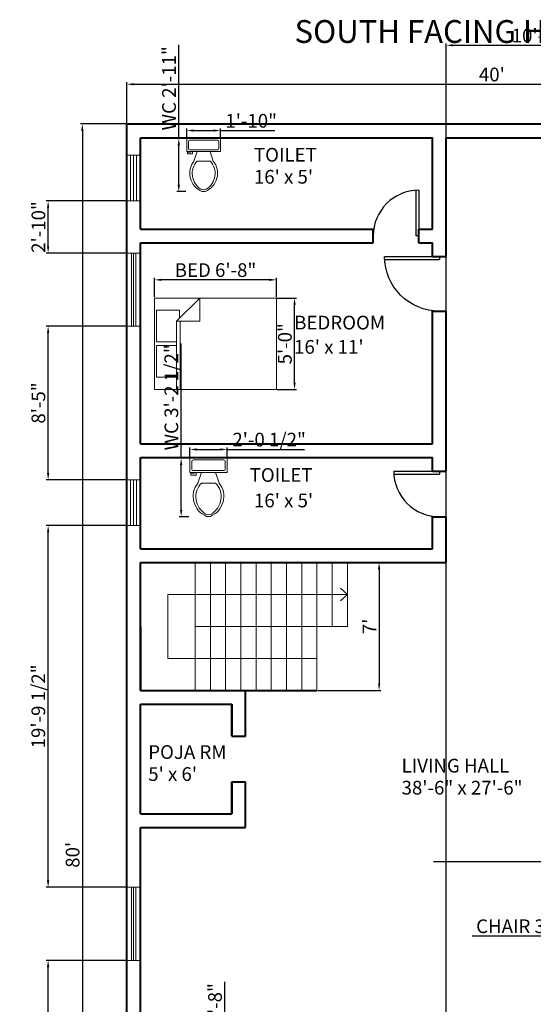
# Model space of a CAD drawing. Units: inches. Extents: x 2383 to 6214, y 970 to 3250.
# Tile 3 of 4: x 2383 to 2721, y 1500 to 2147. Entities that reach past the tile are written whole.
import ezdxf

# ---------------------------------------------------------------- set-up
doc = ezdxf.new("R2010")
doc.units = ezdxf.units.IN
for name, color, linetype, lineweight in [('A-ANNO-DIMS', 2, 'Continuous', 18), ('A-ANNO-TEXT', 7, 'Continuous', 18), ('A-AREA-IDEN', 7, 'Continuous', 18), ('A-DOOR', 4, 'Continuous', 25), ('A-FLOR-FIXT', 8, 'Continuous', 18), ('A-FLOR-STRS', 7, 'Continuous', 20), ('A-FURN', 8, 'Continuous', 18), ('A-GLAZ', 4, 'Continuous', 18), ('A-WALL', 7, 'Continuous', 40)]:
    doc.layers.add(name, color=color, linetype=linetype, lineweight=lineweight)
doc.styles.get("Standard").update_dxf_attribs({"font": 'arial.ttf'})
doc.dimstyles.new('ISO-25', dxfattribs={"dimtxt": 9, "dimasz": 4.5, "dimexe": 1.25, "dimexo": 0.625, "dimtad": 1, "dimdec": 0, "dimlunit": 3, "dimtxsty": 'Standard', "dimcen": 2.5, "dimadec": 0, "dimazin": 0, "dimtfac": 1, "dimtdec": 0, "dimtmove": 0, "dimatfit": 3, "dimfxl": 1, "dimarcsym": 0})

# ---------------------------------------------------------------- blocks, each defined once
blk = doc.blocks.new('Toilet - top')
for p, q in [((9.5, -6), (9.5, -2)), ((-10, -8.5), (-8, -8.5)), ((-10, -9.5), (-10, -8.5)), ((-7, -9.5), (-10, -9.5)), ((-8, -8.5), (-8, -8)), ((-7, -8), (-7, -9.5)), ((-4, -8), (-6, -14)), ((4, -8), (6, -14)), ((4, -14), (-4, -14))]:
    blk.add_line(p, q)
blk.add_lwpolyline([(10.5, -8), (10.5, 0), (-10.5, 0), (-10.5, -8)], close=True)
for points in [[(-9.5, -2), (-9.5, -6)], [(8.5, -1), (-8.5, -1)], [(-8.5, -7), (8.5, -7)]]:
    blk.add_lwpolyline(points)
for centre, radius, start, end in [((-8.62, -1.88), 0.884, 81.8699, 188.1301), ((8.62, -1.88), 0.884, 351.8699, 98.1301), ((-8.62, -6.12), 0.884, 171.8699, 278.1301), ((8.62, -6.12), 0.884, 261.8699, 8.1301), ((3.52, -21.58), 12.17, 141.4691, 247.9714), ((4.2, -21.82), 11.33, 136.3677, 238.9468), ((-3.52, -21.58), 12.17, 292.0284, 38.5307), ((-4.2, -21.82), 11.33, 301.053, 43.6321), ((0, -27.88), 4, 245.7318, 294.2682), ((0, -29), 4, 254.8605, 285.1395)]:
    blk.add_arc(centre, radius, start, end)
blk = doc.blocks.new('Bed - Queen')
for p, q in [((0, -80.00003), (0, 0)), ((0, 0), (59.99999, 0)), ((59.99999, 0), (59.99999, -80.00003)), ((7.99999, -1.2), (28.79998, -1.2)), ((7.99999, -14.4), (7.99999, -1.2)), ((28.79998, -1.2), (28.79998, -14.4)), ((31.19999, -1.2), (51.99999, -1.2)), ((31.19999, -14.4), (31.19999, -1.2)), ((51.99999, -1.2), (51.99999, -16.4)), ((0, -14.4), (44.8, -14.4)), ((44.8, -16.8), (0, -16.8)), ((59.99999, -29.6), (44.8, -14.4)), ((44.8, -14.4), (44.8, -29.6)), ((51.99999, -16.4), (46.79936, -16.4)), ((44.8, -29.6), (59.99999, -29.6)), ((59.99999, -80.00003), (0, -80.00003))]:
    blk.add_line(p, q)
blk = doc.blocks.new('*D14')
at = {"layer": 'A-ANNO-DIMS', "color": 0, "lineweight": -2, "transparency": 16777216}
for p, q in [((2453.83, 2079.3), (2453.83, 2106.04)), ((2458.33, 2104.79), (2929.33, 2104.79)), ((2933.83, 2079.3), (2933.83, 2106.04))]:
    blk.add_line(p, q, dxfattribs=at)
at = {"layer": 'A-ANNO-DIMS', "color": 0, "transparency": 16777216}
for points in [[(2458.33, 2105.54), (2458.33, 2104.04), (2453.83, 2104.79)], [(2929.33, 2105.54), (2929.33, 2104.04), (2933.83, 2104.79)]]:
    blk.add_solid(points, dxfattribs=at)
at = {"layer": 'Defpoints', "color": 0, "transparency": 16777216}
for p in [(2933.83, 2104.79), (2453.83, 2078.68), (2933.83, 2078.68)]:
    blk.add_point(p, dxfattribs=at)
at = {"layer": 'A-ANNO-DIMS', "color": 0, "transparency": 16777216, "insert": (2693.83, 2110.01), "char_height": 9, "attachment_point": 5}
blk.add_mtext("40'", dxfattribs=at)
blk = doc.blocks.new('*D15')
at = {"layer": 'A-ANNO-DIMS', "color": 0, "lineweight": -2, "transparency": 16777216}
for p, q in [((2599.45, 1790.68), (2620.95, 1790.68)), ((2619.7, 1786.18), (2619.7, 1711.18)), ((2579.45, 1706.68), (2620.95, 1706.68))]:
    blk.add_line(p, q, dxfattribs=at)
at = {"layer": 'A-ANNO-DIMS', "color": 0, "transparency": 16777216}
for points in [[(2618.95, 1786.18), (2620.45, 1786.18), (2619.7, 1790.68)], [(2618.95, 1711.18), (2620.45, 1711.18), (2619.7, 1706.68)]]:
    blk.add_solid(points, dxfattribs=at)
at = {"layer": 'Defpoints', "color": 0, "transparency": 16777216}
for p in [(2598.83, 1790.68), (2578.83, 1706.68), (2619.7, 1706.68)]:
    blk.add_point(p, dxfattribs=at)
at = {"layer": 'A-ANNO-DIMS', "color": 0, "transparency": 16777216, "insert": (2614.57, 1748.68), "char_height": 9, "attachment_point": 5, "rotation": 90}
blk.add_mtext("7'", dxfattribs=at)
blk = doc.blocks.new('*D16')
at = {"layer": 'A-ANNO-DIMS', "color": 0, "lineweight": -2, "transparency": 16777216}
for p, q in [((2453.2, 2078.68), (2423.38, 2078.68)), ((2424.63, 2074.18), (2424.63, 1123.18)), ((2453.2, 1118.68), (2423.38, 1118.68))]:
    blk.add_line(p, q, dxfattribs=at)
at = {"layer": 'A-ANNO-DIMS', "color": 0, "transparency": 16777216}
for points in [[(2423.88, 2074.18), (2425.38, 2074.18), (2424.63, 2078.68)], [(2423.88, 1123.18), (2425.38, 1123.18), (2424.63, 1118.68)]]:
    blk.add_solid(points, dxfattribs=at)
at = {"layer": 'Defpoints', "color": 0, "transparency": 16777216}
for p in [(2453.83, 2078.68), (2424.63, 1118.68), (2453.83, 1118.68)]:
    blk.add_point(p, dxfattribs=at)
at = {"layer": 'A-ANNO-DIMS', "color": 0, "transparency": 16777216, "insert": (2419.41, 1598.68), "char_height": 9, "attachment_point": 5, "rotation": 90}
blk.add_mtext("80'", dxfattribs=at)
blk = doc.blocks.new('DOOR-SWING-36IN')
for p, q in [((36, 36), (0, 36)), ((0, 36), (0, 34)), ((36, 34), (0, 34))]:
    blk.add_line(p, q)
blk.add_arc((0, 36), 36, 270, 0)
blk = doc.blocks.new('DOOR-SWING-30IN')
for p, q in [((28, 30), (28, 0)), ((30, 30), (30, 0)), ((30, 0), (28, 0))]:
    blk.add_line(p, q)
blk.add_arc((30, 0), 30, 90, 180)
blk = doc.blocks.new('WINDOW-48X9IN')
for p, q in [((3, 0), (3, 48)), ((4.5, 0), (4.5, 48)), ((6, 0), (6, 48))]:
    blk.add_line(p, q)
blk.add_lwpolyline([(0, 0), (0, 48), (9, 48), (9, 0)], close=True)
blk = doc.blocks.new('VENTILATOR-30X9IN')
for p, q in [((0, 0), (0, 30)), ((0, 30), (9, 30)), ((2.5, 0), (2.5, 30)), ((4.5, 0), (4.5, 30)), ((6.5, 0), (6.5, 30)), ((9, 30), (9, 0)), ((9, 0), (0, 0))]:
    blk.add_line(p, q)
blk = doc.blocks.new('*D23')
at = {"layer": 'A-ANNO-DIMS', "color": 0, "lineweight": -2, "transparency": 16777216}
for p, q in [((2472.15, 1964.96), (2472.15, 1977.58)), ((2547.65, 1976.33), (2476.65, 1976.33)), ((2552.15, 1964.96), (2552.15, 1977.58))]:
    blk.add_line(p, q, dxfattribs=at)
at = {"layer": 'A-ANNO-DIMS', "color": 0, "transparency": 16777216}
for points in [[(2476.65, 1977.08), (2476.65, 1975.58), (2472.15, 1976.33)], [(2547.65, 1977.08), (2547.65, 1975.58), (2552.15, 1976.33)]]:
    blk.add_solid(points, dxfattribs=at)
at = {"layer": 'Defpoints', "color": 0, "transparency": 16777216}
for p in [(2472.15, 1976.33), (2472.15, 1964.33), (2552.15, 1964.33)]:
    blk.add_point(p, dxfattribs=at)
at = {"layer": 'A-ANNO-DIMS', "color": 0, "transparency": 16777216, "insert": (2512.15, 1981.55), "char_height": 9, "attachment_point": 5}
blk.add_mtext('BED 6\'-8"', dxfattribs=at)
blk = doc.blocks.new('*D24')
at = {"layer": 'A-ANNO-DIMS', "color": 0, "lineweight": -2, "transparency": 16777216}
for p, q in [((2552.78, 1964.33), (2565.4, 1964.33)), ((2564.15, 1908.83), (2564.15, 1959.83)), ((2552.78, 1904.33), (2565.4, 1904.33))]:
    blk.add_line(p, q, dxfattribs=at)
at = {"layer": 'A-ANNO-DIMS', "color": 0, "transparency": 16777216}
for points in [[(2563.4, 1959.83), (2564.9, 1959.83), (2564.15, 1964.33)], [(2563.4, 1908.83), (2564.9, 1908.83), (2564.15, 1904.33)]]:
    blk.add_solid(points, dxfattribs=at)
at = {"layer": 'Defpoints', "color": 0, "transparency": 16777216}
for p in [(2552.15, 1964.33), (2564.15, 1964.33), (2552.15, 1904.33)]:
    blk.add_point(p, dxfattribs=at)
at = {"layer": 'A-ANNO-DIMS', "color": 0, "transparency": 16777216, "insert": (2558.93, 1934.33), "char_height": 9, "attachment_point": 5, "rotation": 90}
blk.add_mtext('5\'-0"', dxfattribs=at)
blk = doc.blocks.new('*D31')
at = {"layer": 'A-ANNO-DIMS', "color": 0, "lineweight": -2, "transparency": 16777216}
for p, q in [((2489.58, 1859.16), (2489.58, 1934.61)), ((2494.72, 1859.16), (2488.33, 1859.16)), ((2489.58, 1825.22), (2489.58, 1854.66)), ((2494.72, 1820.72), (2488.33, 1820.72))]:
    blk.add_line(p, q, dxfattribs=at)
at = {"layer": 'A-ANNO-DIMS', "color": 0, "transparency": 16777216}
for points in [[(2488.83, 1854.66), (2490.33, 1854.66), (2489.58, 1859.16)], [(2488.83, 1825.22), (2490.33, 1825.22), (2489.58, 1820.72)]]:
    blk.add_solid(points, dxfattribs=at)
at = {"layer": 'Defpoints', "color": 0, "transparency": 16777216}
for p in [(2489.58, 1859.16), (2495.34, 1859.16), (2495.34, 1820.72)]:
    blk.add_point(p, dxfattribs=at)
at = {"layer": 'A-ANNO-DIMS', "color": 0, "transparency": 16777216, "insert": (2484.3, 1899.14), "char_height": 9, "attachment_point": 5, "rotation": 90}
blk.add_mtext('WC 3\'-2 1/2"', dxfattribs=at)
blk = doc.blocks.new('*D32')
at = {"layer": 'A-ANNO-DIMS', "color": 0, "lineweight": -2, "transparency": 16777216}
for p, q in [((2495.34, 1859.78), (2495.34, 1866.17)), ((2499.84, 1864.92), (2515.27, 1864.92)), ((2519.77, 1859.78), (2519.77, 1866.17)), ((2519.77, 1864.92), (2570.57, 1864.92))]:
    blk.add_line(p, q, dxfattribs=at)
at = {"layer": 'A-ANNO-DIMS', "color": 0, "transparency": 16777216}
for points in [[(2499.84, 1865.67), (2499.84, 1864.17), (2495.34, 1864.92)], [(2515.27, 1865.67), (2515.27, 1864.17), (2519.77, 1864.92)]]:
    blk.add_solid(points, dxfattribs=at)
at = {"layer": 'Defpoints', "color": 0, "transparency": 16777216}
for p in [(2519.77, 1864.92), (2495.34, 1859.16), (2519.77, 1859.16)]:
    blk.add_point(p, dxfattribs=at)
at = {"layer": 'A-ANNO-DIMS', "color": 0, "transparency": 16777216, "insert": (2547.42, 1870.2), "char_height": 9, "attachment_point": 5}
blk.add_mtext('2\'-0 1/2"', dxfattribs=at)
blk = doc.blocks.new('*D33')
at = {"layer": 'A-ANNO-DIMS', "color": 0, "lineweight": -2, "transparency": 16777216}
for p, q in [((2488.03, 2069.14), (2488.03, 2130.62)), ((2492.64, 2069.14), (2486.78, 2069.14)), ((2488.03, 2038.74), (2488.03, 2064.64)), ((2492.64, 2034.24), (2486.78, 2034.24))]:
    blk.add_line(p, q, dxfattribs=at)
at = {"layer": 'A-ANNO-DIMS', "color": 0, "transparency": 16777216}
for points in [[(2487.28, 2064.64), (2488.78, 2064.64), (2488.03, 2069.14)], [(2487.28, 2038.74), (2488.78, 2038.74), (2488.03, 2034.24)]]:
    blk.add_solid(points, dxfattribs=at)
at = {"layer": 'Defpoints', "color": 0, "transparency": 16777216}
for p in [(2488.03, 2069.14), (2493.27, 2069.14), (2493.27, 2034.24)]:
    blk.add_point(p, dxfattribs=at)
at = {"layer": 'A-ANNO-DIMS', "color": 0, "transparency": 16777216, "insert": (2482.76, 2102.13), "char_height": 9, "attachment_point": 5, "rotation": 90}
blk.add_mtext('WC 2\'-11"', dxfattribs=at)
blk = doc.blocks.new('*D34')
at = {"layer": 'A-ANNO-DIMS', "color": 0, "lineweight": -2, "transparency": 16777216}
for p, q in [((2493.27, 2069.77), (2493.27, 2075.63)), ((2497.77, 2074.38), (2510.95, 2074.38)), ((2515.45, 2069.77), (2515.45, 2075.63)), ((2515.45, 2074.38), (2551.27, 2074.38))]:
    blk.add_line(p, q, dxfattribs=at)
at = {"layer": 'A-ANNO-DIMS', "color": 0, "transparency": 16777216}
for points in [[(2497.77, 2075.13), (2497.77, 2073.63), (2493.27, 2074.38)], [(2510.95, 2075.13), (2510.95, 2073.63), (2515.45, 2074.38)]]:
    blk.add_solid(points, dxfattribs=at)
at = {"layer": 'Defpoints', "color": 0, "transparency": 16777216}
for p in [(2515.45, 2074.38), (2493.27, 2069.14), (2515.45, 2069.14)]:
    blk.add_point(p, dxfattribs=at)
at = {"layer": 'A-ANNO-DIMS', "color": 0, "transparency": 16777216, "insert": (2535.61, 2079.6), "char_height": 9, "attachment_point": 5}
blk.add_mtext('1\'-10"', dxfattribs=at)
blk = doc.blocks.new('*D35')
at = {"layer": 'A-ANNO-DIMS', "color": 0, "lineweight": -2, "transparency": 16777216}
for p, q in [((2518.27, 1460.68), (2518.27, 1515.16)), ((2512.31, 1460.68), (2519.52, 1460.68)), ((2518.27, 1421.25), (2518.27, 1456.18)), ((2512.31, 1416.75), (2519.52, 1416.75))]:
    blk.add_line(p, q, dxfattribs=at)
at = {"layer": 'A-ANNO-DIMS', "color": 0, "transparency": 16777216}
for points in [[(2517.52, 1456.18), (2519.02, 1456.18), (2518.27, 1460.68)], [(2517.52, 1421.25), (2519.02, 1421.25), (2518.27, 1416.75)]]:
    blk.add_solid(points, dxfattribs=at)
at = {"layer": 'Defpoints', "color": 0, "transparency": 16777216}
for p in [(2511.68, 1460.68), (2518.27, 1460.68), (2511.68, 1416.75)]:
    blk.add_point(p, dxfattribs=at)
at = {"layer": 'A-ANNO-DIMS', "color": 0, "transparency": 16777216, "insert": (2512.99, 1490.17), "char_height": 9, "attachment_point": 5, "rotation": 90}
blk.add_mtext('WC 3\'-8"', dxfattribs=at)
blk = doc.blocks.new('*D37')
at = {"layer": 'A-ANNO-DIMS', "color": 0, "lineweight": -2, "transparency": 16777216}
for p, q in [((2783.96, 1539.97), (2783.96, 1546.56)), ((2823.73, 1539.97), (2823.73, 1546.56)), ((2783.96, 1545.31), (2680.84, 1545.31)), ((2819.23, 1545.31), (2788.46, 1545.31))]:
    blk.add_line(p, q, dxfattribs=at)
at = {"layer": 'A-ANNO-DIMS', "color": 0, "transparency": 16777216}
for points in [[(2788.46, 1546.06), (2788.46, 1544.56), (2783.96, 1545.31)], [(2819.23, 1546.06), (2819.23, 1544.56), (2823.73, 1545.31)]]:
    blk.add_solid(points, dxfattribs=at)
at = {"layer": 'Defpoints', "color": 0, "transparency": 16777216}
for p in [(2783.96, 1545.31), (2783.96, 1539.35), (2823.73, 1539.35)]:
    blk.add_point(p, dxfattribs=at)
at = {"layer": 'A-ANNO-DIMS', "color": 0, "transparency": 16777216, "insert": (2730.15, 1550.6), "char_height": 9, "attachment_point": 5}
blk.add_mtext('CHAIR 3\'-4" TYP.', dxfattribs=at)
blk = doc.blocks.new('*D56')
at = {"layer": 'A-ANNO-DIMS', "color": 0, "lineweight": -2, "transparency": 16777216}
for p, q in [((2663.83, 1128.3), (2663.83, 2131.63)), ((2668.33, 2130.38), (2779.33, 2130.38)), ((2783.83, 1128.3), (2783.83, 2131.63))]:
    blk.add_line(p, q, dxfattribs=at)
at = {"layer": 'A-ANNO-DIMS', "color": 0, "transparency": 16777216}
for points in [[(2668.33, 2131.13), (2668.33, 2129.63), (2663.83, 2130.38)], [(2779.33, 2131.13), (2779.33, 2129.63), (2783.83, 2130.38)]]:
    blk.add_solid(points, dxfattribs=at)
at = {"layer": 'Defpoints', "color": 0, "transparency": 16777216}
for p in [(2783.83, 2130.38), (2663.83, 1127.68), (2783.83, 1127.68)]:
    blk.add_point(p, dxfattribs=at)
at = {"layer": 'A-ANNO-DIMS', "color": 0, "transparency": 16777216, "insert": (2723.83, 2135.6), "char_height": 9, "attachment_point": 5}
blk.add_mtext('10\'-0"', dxfattribs=at)
blk = doc.blocks.new('*D61')
at = {"layer": 'A-ANNO-DIMS', "color": 0, "lineweight": -2, "transparency": 16777216}
for p, q in [((2453.2, 1529.36), (2400.88, 1529.36)), ((2402.13, 1381.93), (2402.13, 1524.86)), ((2453.2, 1377.43), (2400.88, 1377.43))]:
    blk.add_line(p, q, dxfattribs=at)
at = {"layer": 'A-ANNO-DIMS', "color": 0, "transparency": 16777216}
for points in [[(2401.38, 1524.86), (2402.88, 1524.86), (2402.13, 1529.36)], [(2401.38, 1381.93), (2402.88, 1381.93), (2402.13, 1377.43)]]:
    blk.add_solid(points, dxfattribs=at)
at = {"layer": 'Defpoints', "color": 0, "transparency": 16777216}
for p in [(2402.13, 1529.36), (2453.83, 1529.36), (2453.83, 1377.43)]:
    blk.add_point(p, dxfattribs=at)
at = {"layer": 'A-ANNO-DIMS', "color": 0, "transparency": 16777216, "insert": (2396.91, 1453.4), "char_height": 9, "attachment_point": 5, "rotation": 90}
blk.add_mtext('12\'-8"', dxfattribs=at)
blk = doc.blocks.new('*D62')
at = {"layer": 'A-ANNO-DIMS', "color": 0, "lineweight": -2, "transparency": 16777216}
for p, q in [((2453.2, 1814.95), (2400.88, 1814.95)), ((2402.13, 1581.86), (2402.13, 1810.45)), ((2453.2, 1577.36), (2400.88, 1577.36))]:
    blk.add_line(p, q, dxfattribs=at)
at = {"layer": 'A-ANNO-DIMS', "color": 0, "transparency": 16777216}
for points in [[(2401.38, 1810.45), (2402.88, 1810.45), (2402.13, 1814.95)], [(2401.38, 1581.86), (2402.88, 1581.86), (2402.13, 1577.36)]]:
    blk.add_solid(points, dxfattribs=at)
at = {"layer": 'Defpoints', "color": 0, "transparency": 16777216}
for p in [(2402.13, 1814.95), (2453.83, 1814.95), (2453.83, 1577.36)]:
    blk.add_point(p, dxfattribs=at)
at = {"layer": 'A-ANNO-DIMS', "color": 0, "transparency": 16777216, "insert": (2396.85, 1696.16), "char_height": 9, "attachment_point": 5, "rotation": 90}
blk.add_mtext('19\'-9 1/2"', dxfattribs=at)
blk = doc.blocks.new('*D63')
at = {"layer": 'A-ANNO-DIMS', "color": 0, "lineweight": -2, "transparency": 16777216}
for p, q in [((2453.2, 1945.91), (2400.88, 1945.91)), ((2402.13, 1849.45), (2402.13, 1941.41)), ((2453.2, 1844.95), (2400.88, 1844.95))]:
    blk.add_line(p, q, dxfattribs=at)
at = {"layer": 'A-ANNO-DIMS', "color": 0, "transparency": 16777216}
for points in [[(2401.38, 1941.41), (2402.88, 1941.41), (2402.13, 1945.91)], [(2401.38, 1849.45), (2402.88, 1849.45), (2402.13, 1844.95)]]:
    blk.add_solid(points, dxfattribs=at)
at = {"layer": 'Defpoints', "color": 0, "transparency": 16777216}
for p in [(2402.13, 1945.91), (2453.83, 1945.91), (2453.83, 1844.95)]:
    blk.add_point(p, dxfattribs=at)
at = {"layer": 'A-ANNO-DIMS', "color": 0, "transparency": 16777216, "insert": (2396.91, 1895.43), "char_height": 9, "attachment_point": 5, "rotation": 90}
blk.add_mtext('8\'-5"', dxfattribs=at)
blk = doc.blocks.new('*D64')
at = {"layer": 'A-ANNO-DIMS', "color": 0, "lineweight": -2, "transparency": 16777216}
for p, q in [((2453.2, 2028.12), (2400.88, 2028.12)), ((2402.13, 1998.41), (2402.13, 2023.62)), ((2453.2, 1993.91), (2400.88, 1993.91))]:
    blk.add_line(p, q, dxfattribs=at)
at = {"layer": 'A-ANNO-DIMS', "color": 0, "transparency": 16777216}
for points in [[(2401.38, 2023.62), (2402.88, 2023.62), (2402.13, 2028.12)], [(2401.38, 1998.41), (2402.88, 1998.41), (2402.13, 1993.91)]]:
    blk.add_solid(points, dxfattribs=at)
at = {"layer": 'Defpoints', "color": 0, "transparency": 16777216}
for p in [(2402.13, 2028.12), (2453.83, 2028.12), (2453.83, 1993.91)]:
    blk.add_point(p, dxfattribs=at)
at = {"layer": 'A-ANNO-DIMS', "color": 0, "transparency": 16777216, "insert": (2396.91, 2011.01), "char_height": 9, "attachment_point": 5, "rotation": 90}
blk.add_mtext('2\'-10"', dxfattribs=at)
blk = doc.blocks.new('*D71')
at = {"layer": 'A-ANNO-DIMS', "color": 0, "lineweight": -2, "transparency": 16777216}
for p, q in [((2655.53, 1594.18), (2891.6, 1594.18)), ((3053.63, 1594.18), (2896.1, 1594.18))]:
    blk.add_line(p, q, dxfattribs=at)
at = {"layer": 'A-ANNO-DIMS', "color": 0, "transparency": 16777216}
blk.add_solid([(2896.1, 1594.93), (2896.1, 1593.43), (2891.6, 1594.18)], dxfattribs=at)
at = {"layer": 'Defpoints', "color": 0, "transparency": 16777216}
for p in [(2655.53, 1594.18), (2891.6, 1594.18)]:
    blk.add_point(p, dxfattribs=at)
at = {"layer": 'A-ANNO-DIMS', "color": 0, "transparency": 16777216, "insert": (3033.24, 1599.4), "char_height": 9, "attachment_point": 5, "rotation": 0.00005}
blk.add_mtext('R19\'-8"', dxfattribs=at)
blk = doc.blocks.new('*D72')
at = {"layer": 'A-ANNO-DIMS', "color": 0, "lineweight": -2, "transparency": 16777216}
for p, q in [((2680.75, 1594.18), (2903.29, 1594.18)), ((3067.69, 1594.18), (2907.79, 1594.18))]:
    blk.add_line(p, q, dxfattribs=at)
at = {"layer": 'A-ANNO-DIMS', "color": 0, "transparency": 16777216}
blk.add_solid([(2907.79, 1594.93), (2907.79, 1593.43), (2903.29, 1594.18)], dxfattribs=at)
at = {"layer": 'Defpoints', "color": 0, "transparency": 16777216}
for p in [(2680.75, 1594.18), (2903.29, 1594.18)]:
    blk.add_point(p, dxfattribs=at)
at = {"layer": 'A-ANNO-DIMS', "color": 0, "transparency": 16777216, "insert": (3036.81, 1599.46), "char_height": 9, "attachment_point": 5, "rotation": 0.00005}
blk.add_mtext('R18\'-6 1/2"', dxfattribs=at)

msp = doc.modelspace()

# ---------------------------------------------------------------- linework, layer by layer
at = {"layer": 'A-FLOR-STRS'}
for p, q in [((2498.83, 1706.68), (2498.83, 1790.68)), ((2508.83, 1706.68), (2508.83, 1790.68)), ((2518.83, 1706.68), (2518.83, 1790.68)), ((2528.83, 1706.68), (2528.83, 1790.68)), ((2538.83, 1706.68), (2538.83, 1790.68)), ((2548.83, 1706.68), (2548.83, 1790.68)), ((2558.83, 1706.68), (2558.83, 1790.68)), ((2568.83, 1706.68), (2568.83, 1790.68)), ((2578.83, 1706.68), (2578.83, 1790.68)), ((2588.83, 1748.68), (2588.83, 1790.68)), ((2598.83, 1748.68), (2598.83, 1790.68)), ((2598.83, 1769.68), (2594.43, 1773.85)), ((2480.83, 1727.68), (2480.83, 1769.68)), ((2480.83, 1769.68), (2598.83, 1769.68)), ((2598.83, 1769.68), (2594.43, 1765.51)), ((2498.83, 1748.68), (2598.83, 1748.68)), ((2480.83, 1727.68), (2578.83, 1727.68))]:
    msp.add_line(p, q, dxfattribs=at)
at = {"layer": 'A-WALL'}
for p, q in [((2453.83, 2078.68), (2933.83, 2078.68)), ((2453.83, 1118.68), (2453.83, 2078.68)), ((2462.83, 2069.68), (2654.83, 2069.68)), ((2462.83, 2009.68), (2462.83, 2069.68)), ((2654.83, 2009.68), (2654.83, 2069.68)), ((2663.83, 1991.68), (2663.83, 2069.68)), ((2663.83, 2069.68), (2783.83, 2069.68)), ((2462.83, 2009.68), (2615.83, 2009.68)), ((2615.83, 2000.68), (2615.83, 2009.68)), ((2645.83, 2009.68), (2654.83, 2009.68)), ((2645.83, 2000.68), (2645.83, 2009.68)), ((2462.83, 2000.68), (2615.83, 2000.68)), ((2462.83, 1868.68), (2462.83, 2000.68)), ((2645.83, 2000.68), (2654.83, 2000.68)), ((2654.83, 1991.68), (2654.83, 2000.68)), ((2654.83, 1991.68), (2663.83, 1991.68)), ((2654.83, 1955.68), (2663.83, 1955.68)), ((2654.83, 1868.68), (2654.83, 1955.68)), ((2663.83, 1850.68), (2663.83, 1955.68)), ((2462.83, 1868.68), (2654.83, 1868.68)), ((2462.83, 1859.68), (2654.83, 1859.68)), ((2462.83, 1799.68), (2462.83, 1859.68)), ((2654.83, 1850.68), (2654.83, 1859.68)), ((2654.83, 1850.68), (2663.83, 1850.68)), ((2654.83, 1799.68), (2654.83, 1820.68)), ((2654.83, 1820.68), (2663.83, 1820.68)), ((2663.83, 1790.68), (2663.83, 1820.68)), ((2462.83, 1799.68), (2654.83, 1799.68)), ((2462.83, 1790.68), (2663.83, 1790.68)), ((2462.83, 1706.68), (2462.83, 1790.68)), ((2462.83, 1748.68), (2462.83, 1706.68)), ((2462.83, 1706.68), (2578.83, 1706.68)), ((2531.83, 1676.68), (2531.83, 1706.68)), ((2462.83, 1697.68), (2522.83, 1697.68)), ((2462.83, 1625.68), (2462.83, 1697.68)), ((2522.83, 1697.68), (2522.83, 1676.68)), ((2522.83, 1676.68), (2522.83, 1697.68)), ((2522.83, 1676.68), (2531.83, 1676.68)), ((2522.83, 1661.68), (2522.83, 1661.68)), ((2522.83, 1625.68), (2522.83, 1646.68)), ((2522.83, 1646.68), (2531.83, 1646.68)), ((2522.83, 1646.68), (2522.83, 1625.68)), ((2531.83, 1616.68), (2531.83, 1646.68)), ((2462.83, 1625.68), (2522.83, 1625.68)), ((2462.83, 1616.68), (2531.83, 1616.68)), ((2462.83, 1469.68), (2462.83, 1616.68))]:
    msp.add_line(p, q, dxfattribs=at)

# ---------------------------------------------------------------- block references
at = {"layer": 'A-DOOR'}
msp.add_blockref('DOOR-SWING-30IN', (2615.83, 2005.18), dxfattribs=at)
at = {"layer": 'A-DOOR', "extrusion": (0, 0, -1), "zscale": -1}
msp.add_blockref('DOOR-SWING-36IN', (-2659.33, 1955.68), dxfattribs=at)
at = {"layer": 'A-DOOR', "rotation": 90.00000000000088}
msp.add_blockref('DOOR-SWING-30IN', (2659.33, 1820.68), dxfattribs=at)
at = {"layer": 'A-FLOR-FIXT'}
for p, xscale, yscale, zscale in [((2504.36, 2069.14), 1.056044466302133, 1.056044466302133, 1.056044466302133), ((2507.56, 1859.16), 1.163078797238911, 1.163078797238911, 1.163078797238911)]:
    msp.add_blockref('Toilet - top', p, dxfattribs=dict(at, xscale=xscale, yscale=yscale, zscale=zscale))
at = {"layer": 'A-FURN', "rotation": 90}
msp.add_blockref('Bed - Queen', (2472.15, 1904.33), dxfattribs=at)
at = {"layer": 'A-GLAZ'}
for name, p in [('VENTILATOR-30X9IN', (2453.83, 2028.12)), ('WINDOW-48X9IN', (2453.83, 1945.91)), ('VENTILATOR-30X9IN', (2453.83, 1814.95)), ('WINDOW-48X9IN', (2453.83, 1529.36))]:
    msp.add_blockref(name, p, dxfattribs=at)

# ---------------------------------------------------------------- texts
at = {"layer": 'A-ANNO-TEXT'}
msp.add_text('SOUTH FACING HOUSE', height=15, dxfattribs=at).set_placement((2564.12, 2131.92))
at = {"layer": 'A-AREA-IDEN'}
for s, p in [('TOILET ', (2537.41, 2053.96)), ("16' x 5'", (2537.41, 2039.5)), ('BEDROOM', (2563.9, 1943.73)), ("16' x 11'", (2563.81, 1927.79)), ('TOILET ', (2534.62, 1843.65)), ("16' x 5'", (2537.46, 1826.89)), ('POJA RM', (2467.94, 1661.68)), ("5' x 6'", (2467.94, 1647.22)), ('LIVING HALL ', (2634.5, 1652.73)), ('38\'-6" x 27\'-6"', (2634.5, 1638.27))]:
    msp.add_text(s, height=9, dxfattribs=at).set_placement(p)

# ---------------------------------------------------------------- dimensions: what is measured, and where the dimension line sits
at = {"layer": 'A-ANNO-DIMS'}
for base, p1, p2, override, picture, middle in [((2783.83, 2130.38), (2663.83, 1127.68), (2783.83, 1127.68), {"dimdec": 1, "dimlfac": 1, "dimrnd": 0, "dimzin": 1, "dimdsep": 46, "dimlunit": 4, "dimfrac": 2}, '*D56', (2723.83, 2135.6)), ((2933.83, 2104.79), (2453.83, 2078.68), (2933.83, 2078.68), {"dimclrd": 0, "dimclre": 0, "dimclrt": 0}, '*D14', (2693.83, 2110.01)), ((2515.45, 2074.38), (2493.27, 2069.14), (2515.45, 2069.14), {"dimdec": 1, "dimlfac": 1, "dimrnd": 0, "dimzin": 1, "dimdsep": 46, "dimlunit": 4, "dimfrac": 2}, '*D34', (2535.61, 2079.6)), ((2519.77, 1864.92), (2495.34, 1859.16), (2519.77, 1859.16), {"dimdec": 1, "dimlfac": 1, "dimrnd": 0, "dimzin": 1, "dimdsep": 46, "dimlunit": 4, "dimfrac": 2}, '*D32', (2547.42, 1870.2))]:
    dim = msp.add_linear_dim(base=base, p1=p1, p2=p2, dimstyle='ISO-25', override=override, dxfattribs=at)
    dim.commit()
    dim.dimension.update_dxf_attribs({"geometry": picture, "text_midpoint": middle})
for base, p1, p2, angle, text, picture, middle in [((2488.03, 2069.14), (2493.27, 2034.24), (2493.27, 2069.14), 90, 'WC <>', '*D33', (2482.76, 2102.13)), ((2472.15, 1976.33), (2552.15, 1964.33), (2472.15, 1964.33), 180, 'BED <>', '*D23', (2512.15, 1981.55)), ((2489.58, 1859.16), (2495.34, 1820.72), (2495.34, 1859.16), 90, 'WC <>', '*D31', (2484.3, 1899.14)), ((2783.96, 1545.31), (2823.73, 1539.35), (2783.96, 1539.35), 180, 'CHAIR <> TYP.', '*D37', (2730.15, 1550.6)), ((2518.27, 1460.68), (2511.68, 1416.75), (2511.68, 1460.68), 90, 'WC <>', '*D35', (2512.99, 1490.17))]:
    dim = msp.add_linear_dim(base=base, p1=p1, p2=p2, angle=angle, text=text, dimstyle='ISO-25', override={"dimdec": 1, "dimlfac": 1, "dimrnd": 0, "dimzin": 1, "dimdsep": 46, "dimlunit": 4, "dimfrac": 2}, dxfattribs=at)
    dim.commit()
    dim.dimension.update_dxf_attribs({"geometry": picture, "text_midpoint": middle})
for base, p1, p2, override, picture, middle in [((2424.63, 1118.68), (2453.83, 2078.68), (2453.83, 1118.68), {"dimclrd": 0, "dimclre": 0, "dimclrt": 0}, '*D16', (2419.41, 1598.68)), ((2402.13, 2028.12), (2453.83, 1993.91), (2453.83, 2028.12), {"dimdec": 1, "dimlfac": 1, "dimrnd": 0, "dimzin": 1, "dimdsep": 46, "dimlunit": 4, "dimfrac": 2}, '*D64', (2396.91, 2011.01)), ((2564.15, 1964.33), (2552.15, 1904.33), (2552.15, 1964.33), {"dimdec": 1, "dimlfac": 1, "dimrnd": 0, "dimzin": 1, "dimdsep": 46, "dimlunit": 4, "dimfrac": 2}, '*D24', (2558.93, 1934.33)), ((2402.13, 1945.91), (2453.83, 1844.95), (2453.83, 1945.91), {"dimdec": 1, "dimlfac": 1, "dimrnd": 0, "dimzin": 1, "dimdsep": 46, "dimlunit": 4, "dimfrac": 2}, '*D63', (2396.91, 1895.43)), ((2402.13, 1814.95), (2453.83, 1577.36), (2453.83, 1814.95), {"dimdec": 1, "dimlfac": 1, "dimrnd": 0, "dimzin": 1, "dimdsep": 46, "dimlunit": 4, "dimfrac": 2}, '*D62', (2396.85, 1696.16)), ((2619.7, 1706.68), (2598.83, 1790.68), (2578.83, 1706.68), {"dimclrd": 0, "dimclre": 0, "dimclrt": 0}, '*D15', (2614.57, 1748.68)), ((2402.13, 1529.36), (2453.83, 1377.43), (2453.83, 1529.36), {"dimdec": 1, "dimlfac": 1, "dimrnd": 0, "dimzin": 1, "dimdsep": 46, "dimlunit": 4, "dimfrac": 2}, '*D61', (2396.91, 1453.4))]:
    dim = msp.add_linear_dim(base=base, p1=p1, p2=p2, angle=90, dimstyle='ISO-25', override=override, dxfattribs=at)
    dim.commit()
    dim.dimension.update_dxf_attribs({"geometry": picture, "text_midpoint": middle})
for center, mpoint, picture, middle in [((2680.75, 1594.18), (2903.29, 1594.18), '*D72', (3036.81, 1594.18)), ((2655.53, 1594.18), (2891.6, 1594.18), '*D71', (3033.24, 1594.18))]:
    dim = msp.add_radius_dim(center=center, mpoint=mpoint, dimstyle='ISO-25', override={"dimdec": 1, "dimlfac": 1, "dimrnd": 0, "dimzin": 1, "dimdsep": 46, "dimlunit": 4, "dimfrac": 2}, dxfattribs=at)
    dim.commit()
    dim.dimension.update_dxf_attribs({"geometry": picture, "text_midpoint": middle, "dimtype": 164})

doc.saveas('drawing.dxf')
